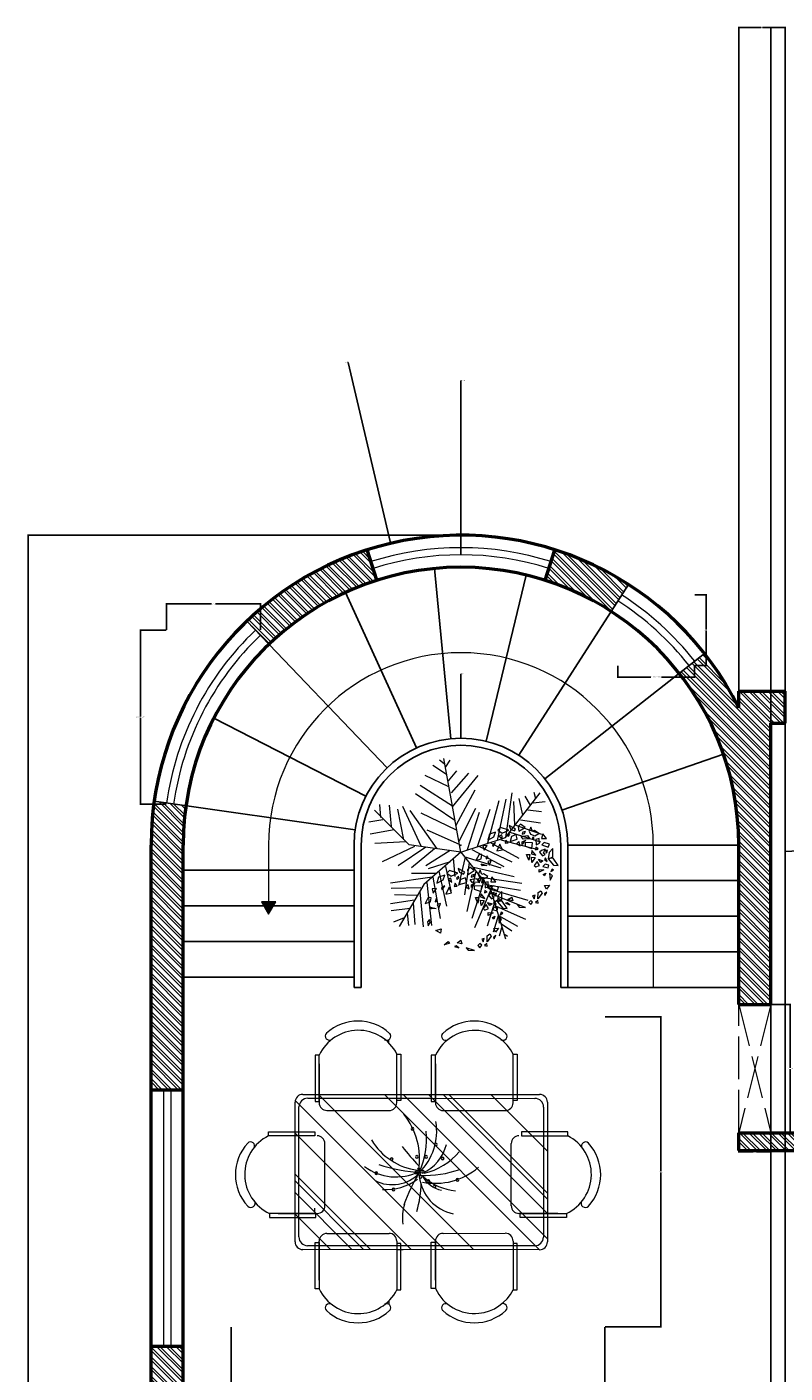
# Model space of a CAD drawing. Units: inches. Extents: x 10696 to 11614, y 5787 to 6498.
# Tile 4 of 9: x 10696 to 10909, y 6120 to 6498. Entities that reach past the tile are written whole.
import ezdxf

# ---------------------------------------------------------------- set-up
doc = ezdxf.new("R2010")
doc.units = ezdxf.units.IN
doc.linetypes.add('ACAD_ISO02W100', pattern=[15, 12, -3])
for name, color, linetype, lineweight in [('A-ANNO-DIMS', 2, 'Continuous', 18), ('A-ANNO-SYMB', 2, 'Continuous', 18), ('A-DOOR', 3, 'Continuous', 25), ('A-FLOR-STRS', 7, 'Continuous', 25), ('A-FURN', 8, 'Continuous', 18), ('A-GLAZ', 4, 'Continuous', 20), ('A-WALL', 7, 'Continuous', 50), ('A-WALL-OVHD', 7, 'ACAD_ISO02W100', 18), ('A-WALL-PATT', 252, 'Continuous', 13), ('L-PLNT', 94, 'Continuous', 13)]:
    doc.layers.add(name, color=color, linetype=linetype, lineweight=lineweight)
doc.styles.get("Standard").update_dxf_attribs({"font": 'arial.ttf'})
doc.dimstyles.get("Standard").update_dxf_attribs({"dimtxt": 0.18, "dimasz": 0.18, "dimexe": 0.18, "dimexo": 0.0625, "dimgap": 0.09, "dimtad": 0, "dimtih": 1, "dimtoh": 1, "dimdec": 4, "dimzin": 0, "dimdsep": 46, "dimtxsty": 'Standard', "dimcen": 0.09, "dimadec": 0, "dimazin": 0, "dimtfac": 1, "dimtdec": 4, "dimtofl": 0, "dimtmove": 0, "dimatfit": 3, "dimfxl": 1, "dimtolj": 1, "dimtzin": 0, "dimarcsym": 0})

# ---------------------------------------------------------------- blocks, each defined once
blk = doc.blocks.new('*U2')
for p, q in [((-8.737, 47.138), (-17.069, 52.711)), ((-10.186, 53.64), (-13.084, 55.962)), ((0, 0), (-10.5, 57)), ((-9.099, 51.782), (-6.563, 55.962)), ((-7.65, 43.423), (-2.578, 49.46)), ((-7.288, 39.707), (-21.778, 46.673)), ((-5.839, 35.992), (4.667, 48.067)), ((-5.114, 27.632), (10.463, 46.673)), ((-3.665, 19.273), (-27.574, 35.527)), ((-5.114, 28.097), (-24.676, 40.636)), ((-2.941, 16.486), (8.652, 37.85)), ((27, 9), (48, 36)), ((27.127, 9.056), (31.112, 35.992)), ((35.096, 32.741), (37.27, 22.524)), ((38.719, 34.134), (41.979, 28.561)), ((44.153, 36.456), (45.239, 32.741)), ((-31.5, 4.5), (-52.5, 25.5)), ((-48.585, 21.131), (-49.309, 29.026)), ((-43.513, 28.561), (-42.427, 15.558)), ((-38.442, 26.239), (-34.819, 7.663)), ((-35.544, 28.097), (-24.314, 3.947)), ((-14.533, 2.09), (-30.834, 25.31)), ((-1.129, 6.734), (9.014, 26.704)), ((10.101, 3.483), (17.708, 26.239)), ((16.259, 5.805), (23.142, 31.348)), ((22.055, 7.198), (27.489, 32.277)), ((31.836, 30.883), (32.561, 16.486)), ((40.53, 25.775), (48.862, 24.846)), ((43.791, 29.954), (51.036, 30.883)), ((-47.498, 19.737), (-55.83, 18.344)), ((-24.314, 23.917), (-2.941, 13.7)), ((3.942, 1.625), (11.187, 24.381)), ((33.285, 16.486), (48.862, 10.913)), ((36.183, 19.737), (48.137, 17.88)), ((-40.615, 13.7), (-55.105, 10.913)), ((-20.691, 13.7), (-1.129, 4.876)), ((0, 0), (27, 9)), ((29.662, 12.307), (48.137, 6.269)), ((-33.37, 6.269), (-52.207, 5.34)), ((-28.299, 3.483), (-47.86, -5.805)), ((-21.416, 3.018), (-38.079, -8.128)), ((0, 0), (-31.5, 4.5)), ((-15.982, 2.09), (-30.11, -9.521)), ((0, 0), (-22.5, -19.5)), ((-6.563, 1.161), (-21.416, -8.128)), ((0, 0), (18, -22.5)), ((6.478, 1.625), (26.04, -8.592)), ((11.187, 3.483), (30.749, -5.805)), ((18.07, 5.805), (35.096, -3.483)), ((24.229, 7.663), (46.688, 1.625)), ((-6.563, -5.805), (-19.967, -9.985)), ((-4.752, -3.483), (-3.665, -14.629)), ((2.493, -3.019), (-1.491, -20.202)), ((1.769, -2.555), (24.229, -9.521)), ((5.029, -6.27), (2.131, -25.775)), ((-17.431, -15.094), (-42.789, -18.809)), ((-15.257, -12.772), (-30.11, -12.772)), ((-17.069, -15.094), (-12.721, -40.172)), ((-13.446, -11.378), (-8.737, -32.741)), ((-9.461, -8.592), (-6.201, -23.453)), ((9.014, -11.378), (3.58, -35.992)), ((7.565, -9.056), (32.198, -14.629)), ((12.274, -15.094), (36.907, -18.809)), ((-24.314, -21.596), (-42.427, -22.06)), ((-22.5, -19.5), (-37.5, -45)), ((-25.038, -23.918), (-22.865, -45.281)), ((-20.691, -18.345), (-17.793, -44.352)), ((14.085, -16.951), (6.478, -40.172)), ((18.07, -22.524), (8.289, -45.745)), ((16.259, -19.738), (36.183, -22.989)), ((18, -22.5), (27, -52.5)), ((18.433, -22.524), (40.53, -29.026)), ((-28.299, -29.026), (-42.789, -31.348)), ((-26.849, -26.24), (-40.253, -25.775)), ((-29.023, -30.884), (-27.936, -43.887)), ((20.244, -30.419), (15.897, -44.816)), ((19.157, -25.311), (38.719, -33.206)), ((-30.834, -34.135), (-42.427, -35.528)), ((-34.457, -39.708), (-40.978, -42.494)), ((-32.646, -36.921), (-31.921, -44.352)), ((22.78, -37.85), (19.519, -48.532)), ((21.331, -32.741), (39.081, -40.636)), ((22.78, -38.314), (34.372, -44.816)), ((24.591, -45.745), (23.142, -50.854)), ((24.591, -43.423), (30.749, -47.603)), ((26.764, -49.925), (28.213, -50.854))]:
    blk.add_line(p, q)
blk = doc.blocks.new('*U3')
for points in [[(-2, 11.66), (-1.6, 10.62), (-0.52, 10.1), (-0.18, 10.62), (-0.79, 10.96)], [(1.24, 12), (0.56, 11.31), (0.76, 10.01), (2.52, 11.05)], [(-5.78, 9.75), (-7.54, 9.23), (-8.01, 7.5), (-6.26, 8.45)], [(-4.43, 11.05), (-5.18, 10.36), (-3.96, 9.49), (-2.07, 10.36)], [(-4.84, 8.63), (-3.83, 7.85), (-4.03, 8.97)], [(-1.94, 9.49), (-2.48, 8.97), (-2.27, 8.54), (-1.8, 9.06)], [(0.02, 9.06), (-1.33, 8.54), (-1.73, 7.16), (0.29, 7.76)], [(1.37, 8.54), (3.13, 8.8), (3.8, 7.85), (1.91, 7.76)], [(2.59, 9.93), (1.84, 9.75), (1.64, 9.23), (2.32, 9.41)], [(4.14, 11.14), (3.6, 10.01), (4, 9.23), (5.22, 8.71), (6.3, 9.41), (5.08, 10.19), (4.61, 10.01)], [(4.61, 8.28), (4.54, 7.76), (4.95, 7.59), (4.95, 8.28)], [(6.43, 7.94), (5.49, 7.68), (5.56, 6.21), (6.5, 6.64)], [(7.45, 9.32), (7.11, 7.94), (8.52, 7.94)], [(-8.14, 6.03), (-9.36, 5.95), (-9.02, 4.73)], [(-5.78, 6.81), (-6.66, 6.21), (-6.52, 5.69)], [(-4.57, 6.38), (-5.45, 4.47), (-3.89, 4.82)], [(-2.88, 7.5), (-3.15, 6.64), (-2.27, 6.72)], [(0.76, 7.16), (0.09, 6.46), (1.1, 5.95)], [(1.71, 6.29), (1.71, 7.07), (2.65, 7.5), (2.11, 6.9)], [(2.52, 6.81), (2.52, 5.86), (4.41, 5.17), (4.61, 6.72)], [(4.41, 4.56), (4.27, 3.7), (5.49, 3.26)], [(5.49, 5.51), (5.42, 4.82), (6.16, 5.08)], [(8.12, 4.99), (7.11, 4.65), (6.5, 4.13), (7.38, 3.09), (8.12, 3.52), (7.65, 3.87)], [(7.85, 6.81), (7.18, 6.21), (9, 5.51), (9.33, 6.38)], [(8.73, 4.73), (8.19, 4.56), (8.39, 3.87), (8.59, 4.04)], [(10.28, 5.17), (9.2, 4.04), (9, 2.31), (10.48, 0.49), (11.76, 0.41), (10.35, 2.48), (9.33, 2.4), (10.28, 2.83)], [(-11.32, 1.79), (-9.83, 2.31), (-9.63, 3.44), (-10.44, 3.52)], [(-8.21, 0.41), (-9.43, 0.32), (-9.83, 0.84)], [(-8.21, 3.09), (-8.48, 2.31), (-7.87, 2.57)], [(-7, 1.79), (-7.94, 1.53), (-7.47, 0.49)], [(3.53, 1.88), (2.86, 3.52), (3.8, 3.52)], [(4.27, 2.74), (5.29, 2.66), (4.41, 1.27)], [(5.83, 1.53), (5.02, 0.41), (5.49, -0.02), (6.5, 0.41)], [(7.51, 1.71), (6.91, 1.27), (6.23, 2.14)], [(8.12, 0.75), (7.51, 0.15), (8.93, -0.28), (9.13, 0.49)], [(8.19, 2.57), (7.92, 2.05), (8.66, 1.53)], [(-10.03, -2.71), (-10.64, -3.31), (-10.44, -4.44), (-9.9, -3.49)], [(7.78, -0.8), (6.43, -1.5), (6.43, -0.72)], [(8.32, -1.75), (7.98, -2.53), (7.58, -2.1)], [(9.33, -1.75), (9.54, -3.74), (10.14, -2.53)], [(10.08, -0.63), (9.74, -1.32), (10.48, -0.89)], [(-8.28, -5.73), (-6.79, -5.3), (-7, -6.51)], [(6.1, -8.94), (6.16, -7.21), (6.91, -6.69), (7.24, -7.38)], [(8.05, -8.07), (8.59, -7.12), (7.92, -7.55)], [(9.33, -5.13), (8.46, -6.25), (7.98, -5.22)], [(-4.84, -8.85), (-4.43, -9.45), (-5.99, -9.8)], [(-2.54, -10.06), (-3.02, -10.23), (-1.8, -10.67)], [(-2.34, -9.2), (-1.26, -8.5), (-0.99, -9.54)], [(0.22, -10.58), (0.83, -11.27), (2.59, -11.36)], [(4.07, -9.45), (3.53, -9.97), (4.07, -10.58), (4.61, -9.89)], [(5.29, -7.98), (4.61, -8.16), (5.02, -8.94)], [(6.03, -9.45), (5.42, -9.97), (6.16, -10.15)]]:
    blk.add_lwpolyline(points, close=True)
blk = doc.blocks.new('A$C6327331B')
for p, q in [((790.8, 678.3), (790.8, 696.4)), ((790.8, 678.3), (790.8, 696.4)), ((1381.3, 692.8), (1381.3, 686.2)), ((1381.3, 692.8), (1381.3, 686.2)), ((410.1, 615.8), (410, 377)), ((410.1, 615.8), (410, 377)), ((431.6, 615.8), (410.1, 615.8)), ((431.6, 615.8), (410.1, 615.8)), ((431.4, 376.9), (431.6, 615.8)), ((431.4, 376.9), (431.6, 615.8)), ((431.5, 571.8), (431.4, 370.8)), ((431.5, 571.8), (431.4, 370.8)), ((831.4, 382.9), (831.6, 621.7)), ((831.4, 382.9), (831.6, 621.7)), ((831.4, 370.6), (831.5, 571.6)), ((831.4, 370.6), (831.5, 571.6)), ((831.6, 621.7), (853, 621.7)), ((831.6, 621.7), (853, 621.7)), ((853, 621.7), (852.9, 382.9)), ((853, 621.7), (852.9, 382.9)), ((1009.3, 615.5), (1009.2, 376.7)), ((1009.3, 615.5), (1009.2, 376.7)), ((1030.7, 615.5), (1009.3, 615.5)), ((1030.7, 615.5), (1009.3, 615.5)), ((1030.6, 376.6), (1030.7, 615.5)), ((1030.6, 376.6), (1030.7, 615.5)), ((1030.7, 571.5), (1030.6, 370.5)), ((1030.7, 571.5), (1030.6, 370.5)), ((1430.6, 382.6), (1430.7, 621.4)), ((1430.6, 382.6), (1430.7, 621.4)), ((1430.6, 370.3), (1430.7, 571.3)), ((1430.6, 370.3), (1430.7, 571.3)), ((1430.7, 621.4), (1452.2, 621.4)), ((1430.7, 621.4), (1452.2, 621.4)), ((1452.2, 621.4), (1452, 382.6)), ((1452.2, 621.4), (1452, 382.6)), ((307.1, -346), (307.5, 374)), ((307.1, -346), (307.5, 374)), ((1075.9, -386.3), (308.5, 383.1)), ((1075.9, -386.3), (308.5, 383.1)), ((327.1, -321), (327.5, 349)), ((347.5, 414), (831.5, 413.8)), ((347.5, 414), (831.5, 413.8)), ((372.5, 394), (831.4, 393.8)), ((372.5, 394), (1009.2, 393.7)), ((410, 377), (431.4, 376.9)), ((410, 377), (431.4, 376.9)), ((1226.3, -386.4), (428, 414)), ((1226.3, -386.4), (428, 414)), ((1567.1, -386.6), (768.8, 413.8)), ((1567.1, -386.6), (768.8, 413.8)), ((852.9, 382.9), (831.4, 382.9)), ((852.9, 382.9), (831.4, 382.9)), ((831.5, 413.8), (1567.5, 413.4)), ((1607.1, -331.3), (864.1, 413.8)), ((1607.1, -331.3), (864.1, 413.8)), ((1607.2, -200.8), (994.4, 413.7)), ((1607.2, -200.8), (994.4, 413.7)), ((1009.2, 413.7), (1567.5, 413.4)), ((1009.2, 393.7), (1542.5, 393.4)), ((1009.2, 376.7), (1030.6, 376.6)), ((1009.2, 376.7), (1030.6, 376.6)), ((1607.2, -125.5), (1069.5, 413.7)), ((1607.2, -125.5), (1069.5, 413.7)), ((1607.2, -95.4), (1099.6, 413.6)), ((1607.2, -95.4), (1099.6, 413.6)), ((1607.3, 120.5), (1315.1, 413.5)), ((1607.3, 120.5), (1315.1, 413.5)), ((1415.7, 413.4), (1415.7, 413.5)), ((1415.7, 413.4), (1415.7, 413.5)), ((1452, 382.6), (1430.6, 382.6)), ((1452, 382.6), (1430.6, 382.6)), ((1587.5, 348.4), (1587.1, -321.6)), ((1607.5, 373.4), (1607.1, -346.6)), ((1607.5, 373.4), (1607.1, -346.6)), ((471.4, 330.8), (791.4, 330.6)), ((471.4, 330.8), (791.4, 330.6)), ((1070.6, 330.5), (1390.6, 330.3)), ((1070.6, 330.5), (1390.6, 330.3)), ((169.9, 221.5), (408.7, 221.6)), ((169.9, 221.5), (408.7, 221.6)), ((169.9, 200.1), (169.9, 221.5)), ((169.9, 200.1), (169.9, 221.5)), ((905.5, -386.3), (307.4, 213.5)), ((905.5, -386.3), (307.4, 213.5)), ((408.7, 221.6), (408.7, 200.2)), ((408.7, 221.6), (408.7, 200.2)), ((1473.3, 221.6), (1473.3, 200.2)), ((1473.3, 221.6), (1473.3, 200.2)), ((1712.1, 221.5), (1473.3, 221.6)), ((1712.1, 221.5), (1473.3, 221.6)), ((1712.1, 200.1), (1712.1, 221.5)), ((1712.1, 200.1), (1712.1, 221.5)), ((408.7, 200.2), (169.9, 200.1)), ((408.7, 200.2), (169.9, 200.1)), ((461.2, -159.8), (461, 160.2)), ((461.2, -159.8), (461, 160.2)), ((1420.8, -159.8), (1420.9, 160.2)), ((1420.8, -159.8), (1420.9, 160.2)), ((1473.3, 200.2), (1712.1, 200.1)), ((1473.3, 200.2), (1712.1, 200.1)), ((695.1, -386.2), (307.3, 2.7)), ((695.1, -386.2), (307.3, 2.7)), ((44.6, -20.2), (44.5, -20.1)), ((44.6, -20.2), (44.5, -20.1)), ((660, -386.1), (307.3, -32.5)), ((660, -386.1), (307.3, -32.5)), ((1837.4, -20.2), (1837.5, -20.1)), ((1837.4, -20.2), (1837.5, -20.1)), ((599.8, -386.1), (307.2, -92.7)), ((599.8, -386.1), (307.2, -92.7)), ((415.1, -199.8), (176.2, -199.9)), ((415.1, -199.8), (176.2, -199.9)), ((176.2, -199.9), (176.2, -221.3)), ((176.2, -199.9), (176.2, -221.3)), ((220.2, -199.9), (421.2, -199.8)), ((220.2, -199.9), (421.2, -199.8)), ((489.6, -386), (307.2, -203.2)), ((489.6, -386), (307.2, -203.2)), ((408.7, -193.6), (408.7, -172.1)), ((408.7, -193.6), (408.7, -172.1)), ((415.1, -221.2), (415.1, -199.8)), ((415.1, -221.2), (415.1, -199.8)), ((1661.8, -199.9), (1460.8, -199.8)), ((1661.8, -199.9), (1460.8, -199.8)), ((1466.9, -221.2), (1466.9, -199.8)), ((1466.9, -221.2), (1466.9, -199.8)), ((1466.9, -199.8), (1705.7, -199.9)), ((1466.9, -199.8), (1705.7, -199.9)), ((1705.7, -199.9), (1705.7, -221.3)), ((1705.7, -199.9), (1705.7, -221.3)), ((176.2, -221.3), (415.1, -221.2)), ((176.2, -221.3), (415.1, -221.2)), ((1705.7, -221.3), (1466.9, -221.2)), ((1705.7, -221.3), (1466.9, -221.2)), ((431.5, -543.7), (431.4, -342.7)), ((431.5, -543.7), (431.4, -342.7)), ((471.4, -302.7), (791.4, -302.5)), ((471.4, -302.7), (791.4, -302.5)), ((831.4, -342.5), (831.5, -543.5)), ((831.4, -342.5), (831.5, -543.5)), ((1030.7, -543.4), (1030.6, -342.4)), ((1030.7, -543.4), (1030.6, -342.4)), ((1070.6, -302.4), (1390.6, -302.2)), ((1070.6, -302.4), (1390.6, -302.2)), ((1430.6, -342.2), (1430.7, -543.2)), ((1430.6, -342.2), (1430.7, -543.2)), ((1567.1, -386.6), (347.1, -386)), ((1567.1, -386.6), (347.1, -386)), ((1542.1, -366.6), (372.1, -366)), ((410.1, -587.7), (410, -348.9)), ((410.1, -587.7), (410, -348.9)), ((410, -348.9), (431.4, -348.9)), ((410, -348.9), (431.4, -348.9)), ((431.4, -348.9), (431.6, -587.7)), ((431.4, -348.9), (431.6, -587.7)), ((831.4, -354.8), (831.6, -593.6)), ((831.4, -354.8), (831.6, -593.6)), ((852.9, -354.8), (831.4, -354.8)), ((852.9, -354.8), (831.4, -354.8)), ((831.5, -385.7), (864.1, -385.7)), ((831.5, -385.7), (864.1, -385.7)), ((853, -593.6), (852.9, -354.8)), ((853, -593.6), (852.9, -354.8)), ((1009.2, -348.6), (1030.6, -348.5)), ((1009.2, -348.6), (1030.6, -348.5)), ((1009.3, -587.4), (1009.2, -348.6)), ((1009.3, -587.4), (1009.2, -348.6)), ((1030.6, -348.5), (1030.7, -587.4)), ((1030.6, -348.5), (1030.7, -587.4)), ((1415.7, -385.3), (1415.7, -385.4)), ((1415.7, -385.3), (1415.7, -385.4)), ((1430.6, -354.5), (1430.7, -593.3)), ((1430.6, -354.5), (1430.7, -593.3)), ((1452, -354.5), (1430.6, -354.5)), ((1452, -354.5), (1430.6, -354.5)), ((1452.2, -593.3), (1452, -354.5)), ((1452.2, -593.3), (1452, -354.5)), ((431.6, -587.7), (410.1, -587.7)), ((431.6, -587.7), (410.1, -587.7)), ((831.6, -593.6), (853, -593.6)), ((831.6, -593.6), (853, -593.6)), ((1030.7, -587.4), (1009.3, -587.4)), ((1030.7, -587.4), (1009.3, -587.4)), ((1430.7, -593.3), (1452.2, -593.3)), ((1430.7, -593.3), (1452.2, -593.3)), ((790.8, -650.2), (790.8, -668.4)), ((790.8, -650.2), (790.8, -668.4)), ((1381.3, -664.7), (1381.3, -658.1)), ((1381.3, -664.7), (1381.3, -658.1))]:
    blk.add_line(p, q)
for centre, radius, start, end in [((631.5, 550.5), 241.3, 47.46915, 132.47205), ((631.5, 550.5), 241.3, 47.46915, 132.47205), ((1230.7, 550.2), 241.3, 47.46915, 132.47205), ((1230.7, 550.2), 241.3, 47.46915, 132.47205), ((633, 521.6), 222.4, 26.76564, 154.93691), ((633, 521.6), 222.4, 26.76564, 154.93691), ((484.3, 714.2), 21.2, 137.64965, 300.34124), ((484.3, 714.2), 21.2, 137.64965, 300.34124), ((779, 714), 21.2, 239.59996, 42.29154), ((779, 714), 21.2, 239.59996, 42.29154), ((1232.2, 521.3), 222.4, 84.42654, 154.93691), ((1232.2, 521.3), 222.4, 84.42654, 154.93691), ((1083.4, 713.9), 21.2, 137.64965, 300.34124), ((1083.4, 713.9), 21.2, 137.64965, 300.34124), ((1232.2, 521.3), 222.4, 26.76564, 84.42654), ((1232.2, 521.3), 222.4, 26.76564, 84.42654), ((1378.1, 713.7), 21.2, 239.59996, 42.29154), ((1378.1, 713.7), 21.2, 239.59996, 42.29154), ((347.5, 374), 40, 89.9706, 179.9706), ((347.5, 374), 40, 89.9706, 179.9706), ((372.5, 349), 45, 89.9706, 179.9706), ((471.4, 370.8), 40, 179.9706, 269.9706), ((471.4, 370.8), 40, 179.9706, 269.9706), ((791.4, 370.6), 40, 269.9706, 359.9706), ((791.4, 370.6), 40, 269.9706, 359.9706), ((1070.6, 370.5), 40, 179.9706, 269.9706), ((1070.6, 370.5), 40, 179.9706, 269.9706), ((1390.6, 370.3), 40, 269.9706, 359.9706), ((1390.6, 370.3), 40, 269.9706, 359.9706), ((1542.5, 348.4), 45, 359.9706, 89.9706), ((1567.5, 373.4), 40, 359.9706, 89.9706), ((1567.5, 373.4), 40, 359.9706, 89.9706), ((574.1, 79.9), 374.6, 351.24958, 38.23328), ((912.6, 235.7), 6.91, 0, 180), ((912.6, 235.7), 6.91, 180, 0), ((737.8, 225), 299.2, 314.48606, 9.37622), ((586.4, 182.9), 398.1, 335.08876, 5.96372), ((241.3, 0.1), 241.3, 137.52795, 222.53085), ((270.2, 1.6), 222.4, 116.82445, 244.99571), ((270.2, 1.6), 222.4, 116.82445, 244.99571), ((77.6, 147.4), 21.2, 329.65876, 132.35035), ((77.6, 147.4), 21.2, 329.65876, 132.35035), ((421, 160.2), 40, 0.0294, 90.0294), ((421, 160.2), 40, 0.0294, 90.0294), ((983.2, 350.8), 331, 211.31505, 262.13779), ((2460.3, 1443.6), 2062.1, 219.04877, 222.6799), ((873.8, 207.8), 219.3, 294.09558, 346.29534), ((1033, 155.9), 6.91, 0, 180), ((1033, 155.9), 6.91, 180, 0), ((1460.9, 160.2), 40, 89.9706, 179.9706), ((1460.9, 160.2), 40, 89.9706, 179.9706), ((1611.7, 1.6), 222.4, 295.00429, 63.17555), ((1611.7, 1.6), 222.4, 295.00429, 63.17555), ((1804.4, 147.4), 21.2, 47.64965, 210.34124), ((1804.4, 147.4), 21.2, 47.64965, 210.34124), ((1640.7, 0.1), 241.3, 317.46915, 42.47205), ((1640.7, 0.1), 241.3, 317.46915, 42.47205), ((805, 79.9), 6.91, 0, 180), ((805, 79.9), 6.91, 180, 0), ((934.8, 91.3), 6.91, 0, 180), ((934.8, 91.3), 6.91, 180, 0), ((897.1, 334.6), 335.6, 283.04524, 319.77663), ((982.3, 91.3), 6.91, 0, 180), ((982.3, 91.3), 6.91, 180, 0), ((1067.8, 83.7), 6.91, 0, 180), ((1067.8, 83.7), 6.91, 180, 0), ((826.9, 258.5), 270.1, 233.32313, 295.76326), ((725.8, 7.7), 6.91, 0, 180), ((725.8, 7.7), 6.91, 180, 0), ((807.8, 143), 194.5, 242.99086, 315.91017), ((985.1, 750.7), 739.8, 250.5249, 267.82437), ((1747.6, -469.5), 933.6, 148.98728, 160.36101), ((931.7, 11.5), 6.91, 0, 180), ((931.7, 11.5), 6.91, 180, 0), ((944.3, 26.7), 6.91, 0, 180), ((944.3, 26.7), 6.91, 180, 0), ((947.5, 3.9), 6.91, 0, 180), ((947.5, 3.9), 6.91, 180, 0), ((970.7, 574.8), 578.8, 268.32856, 288.729), ((966.5, 15.3), 6.91, 0, 180), ((966.5, 15.3), 6.91, 180, 0), ((1030.3, 292.7), 337.4, 258.55155, 310.98153), ((776.7, 191.6), 268.2, 265.87406, 306.95584), ((814.5, -75.9), 6.91, 0, 180), ((392.7, -33), 564.4, 343.85612, 359.11051), ((953.8, -11.3), 6.91, 0, 180), ((953.8, -11.3), 6.91, 180, 0), ((1167.7, 15.7), 221.9, 186.99045, 258.02836), ((1090.6, 62.7), 145.4, 208.89012, 258.45792), ((1166.2, 212.9), 298.2, 228.7581, 263.8624), ((995, -34.1), 6.91, 0, 180), ((995, -34.1), 6.91, 180, 0), ((1026.7, -60.7), 6.91, 0, 180), ((1026.7, -60.7), 6.91, 180, 0), ((1143.8, -26.5), 6.91, 0, 180), ((1143.8, -26.5), 6.91, 180, 0), ((79, -146.7), 22.5, 226.37763, 29.88821), ((79, -146.7), 22.5, 226.37763, 29.88821), ((814.5, -75.9), 6.91, 180, 0), ((1803, -146.7), 22.5, 150.11179, 313.62237), ((1803, -146.7), 22.5, 150.11179, 313.62237), ((421.2, -159.8), 40, 270.0294, 0.0294), ((421.2, -159.8), 40, 270.0294, 0.0294), ((1112.9, -226), 252.6, 162.94564, 186.48138), ((1460.8, -159.8), 40, 179.9706, 269.9706), ((1460.8, -159.8), 40, 179.9706, 269.9706), ((347.1, -346), 40, 179.9706, 269.9706), ((347.1, -346), 40, 179.9706, 269.9706), ((372.1, -321), 45, 179.9706, 269.9706), ((471.4, -342.7), 40, 90.0294, 180.0294), ((471.4, -342.7), 40, 90.0294, 180.0294), ((791.4, -342.5), 40, 0.0294, 90.0294), ((791.4, -342.5), 40, 0.0294, 90.0294), ((1070.6, -342.4), 40, 90.0294, 180.0294), ((1070.6, -342.4), 40, 90.0294, 180.0294), ((1390.6, -342.2), 40, 0.0294, 90.0294), ((1390.6, -342.2), 40, 0.0294, 90.0294), ((1542.1, -321.6), 45, 269.9706, 359.9706), ((1567.1, -346.6), 40, 269.9706, 359.9706), ((1567.1, -346.6), 40, 269.9706, 359.9706), ((633, -493.5), 222.4, 205.06309, 333.23436), ((633, -493.5), 222.4, 205.06309, 333.23436), ((1232.2, -493.2), 222.4, 205.06309, 275.57346), ((1232.2, -493.2), 222.4, 205.06309, 275.57346), ((1232.2, -493.2), 222.4, 275.57346, 333.23436), ((1232.2, -493.2), 222.4, 275.57346, 333.23436), ((484.3, -686.1), 21.2, 59.65876, 222.35035), ((484.3, -686.1), 21.2, 59.65876, 222.35035), ((779, -686), 21.2, 317.70846, 120.40004), ((779, -686), 21.2, 317.70846, 120.40004), ((1083.4, -685.8), 21.2, 59.65876, 222.35035), ((1083.4, -685.8), 21.2, 59.65876, 222.35035), ((1378.1, -685.6), 21.2, 317.70846, 120.40004), ((1378.1, -685.6), 21.2, 317.70846, 120.40004), ((631.5, -522.4), 241.3, 227.52795, 312.53085), ((631.5, -522.4), 241.3, 227.52795, 312.53085), ((1230.7, -522.1), 241.3, 227.52795, 312.53085), ((1230.7, -522.1), 241.3, 227.52795, 312.53085)]:
    blk.add_arc(centre, radius, start, end)
at = {"width": 0.8, "flags": 9}
for tag in ['XSIZE', 'YSIZE']:
    blk.add_attdef(tag, (945.2, 11.4), '', height=0.23, rotation=180, dxfattribs=at)
blk = doc.blocks.new('DOOR-SINGLE-36-KITCHEN')
blk.add_line((0, 36), (0, 0))
blk.add_arc((0, 36), 36, 270, 0)
blk = doc.blocks.new('WIN-GLAZ-72')
for p, q in [((0, 72), (0, 0)), ((2, 72), (2, 0))]:
    blk.add_line(p, q)
blk = doc.blocks.new('WIN-ARC-CROWN')
for radius in [83.5, 81.5]:
    blk.add_arc((25.29, -77.67), radius, 72.3705, 107.6295)
blk = doc.blocks.new('WIN-ARC-WEST')
for radius in [83.5, 81.5]:
    blk.add_arc((82.66, -11.5), radius, 133.6902, 171.8873)
blk = doc.blocks.new('WIN-ARC-EAST')
for radius in [83.5, 81.5]:
    blk.add_arc((-44.03, -50.4), radius, 38.1972, 57.2958)
blk = doc.blocks.new('OPENING-OVHD-36X9')
for p, q in [((0, 0), (0, 36)), ((9, 36), (0, 0)), ((0, 36), (9, 0)), ((9, 0), (9, 36))]:
    blk.add_line(p, q)
blk = doc.blocks.new('STAIR-HANDRAIL-RETURN')
for p, q in [((0, 0), (0, 40)), ((60, 0), (60, 40)), ((2, 0), (0, 0)), ((58, 0), (60, 0))]:
    blk.add_line(p, q)
blk.add_lwpolyline([(2, 0), (2, 40, -1), (58, 40), (58, 0)], format="xyb")
blk.add_arc((30, 40), 30, 0, 180)
blk = doc.blocks.new('*D36')
at = {"layer": 'A-ANNO-DIMS', "color": 0, "lineweight": -2, "transparency": 16777216}
for p, q in [((10753.44, 6132.46), (10753.44, 6116.62)), ((10858.3, 6132.46), (10858.3, 6116.62)), ((10753.62, 6116.8), (10804.52, 6116.8)), ((10858.12, 6116.8), (10807.22, 6116.8))]:
    blk.add_line(p, q, dxfattribs=at)
at = {"layer": 'A-ANNO-DIMS', "color": 0, "transparency": 16777216}
for points in [[(10753.62, 6116.83), (10753.62, 6116.77), (10753.44, 6116.8)], [(10858.12, 6116.83), (10858.12, 6116.77), (10858.3, 6116.8)]]:
    blk.add_solid(points, dxfattribs=at)
at = {"layer": 'Defpoints', "color": 0, "transparency": 16777216}
for p in [(10753.44, 6132.52), (10858.3, 6132.52), (10858.3, 6116.8)]:
    blk.add_point(p, dxfattribs=at)
at = {"layer": 'A-ANNO-DIMS', "color": 0, "transparency": 16777216, "insert": (10805.87, 6116.8), "char_height": 0.18, "attachment_point": 5}
blk.add_mtext('\\A1;DINING SET 105 TYP.', dxfattribs=at)
blk = doc.blocks.new('*D37')
at = {"layer": 'A-ANNO-DIMS', "color": 0, "lineweight": -2, "transparency": 16777216}
for p, q in [((10858.36, 6219.59), (10874.21, 6219.59)), ((10874.03, 6219.41), (10874.03, 6176.24)), ((10874.03, 6132.7), (10874.03, 6175.88)), ((10858.36, 6132.52), (10874.21, 6132.52))]:
    blk.add_line(p, q, dxfattribs=at)
at = {"layer": 'A-ANNO-DIMS', "color": 0, "transparency": 16777216}
for points in [[(10874, 6219.41), (10874.06, 6219.41), (10874.03, 6219.59)], [(10874, 6132.7), (10874.06, 6132.7), (10874.03, 6132.52)]]:
    blk.add_solid(points, dxfattribs=at)
at = {"layer": 'Defpoints', "color": 0, "transparency": 16777216}
for p in [(10858.3, 6219.59), (10874.03, 6219.59), (10858.3, 6132.52)]:
    blk.add_point(p, dxfattribs=at)
at = {"layer": 'A-ANNO-DIMS', "color": 0, "transparency": 16777216, "insert": (10874.03, 6176.06), "char_height": 0.18, "attachment_point": 5}
blk.add_mtext('\\A1;87 TYP.', dxfattribs=at)
blk = doc.blocks.new('*D54')
at = {"layer": 'A-ANNO-DIMS', "color": 0, "lineweight": -2, "transparency": 16777216}
for p, q in [((10735.19, 6328.25), (10727.74, 6328.25)), ((10727.92, 6328.07), (10727.92, 6303.99)), ((10727.92, 6279.55), (10727.92, 6303.62)), ((10735.19, 6279.37), (10727.74, 6279.37))]:
    blk.add_line(p, q, dxfattribs=at)
at = {"layer": 'A-ANNO-DIMS', "color": 0, "transparency": 16777216}
for points in [[(10727.89, 6328.07), (10727.95, 6328.07), (10727.92, 6328.25)], [(10727.89, 6279.55), (10727.95, 6279.55), (10727.92, 6279.37)]]:
    blk.add_solid(points, dxfattribs=at)
at = {"layer": 'Defpoints', "color": 0, "transparency": 16777216}
for p in [(10727.92, 6328.25), (10735.25, 6328.25), (10735.25, 6279.37)]:
    blk.add_point(p, dxfattribs=at)
at = {"layer": 'A-ANNO-DIMS', "color": 0, "transparency": 16777216, "insert": (10727.92, 6303.81), "char_height": 0.18, "attachment_point": 5}
blk.add_mtext('\\A1;CURVED LIGHT 49 TYP.', dxfattribs=at)
blk = doc.blocks.new('*D55')
at = {"layer": 'A-ANNO-DIMS', "color": 0, "lineweight": -2, "transparency": 16777216}
for p, q in [((10735.25, 6328.31), (10735.25, 6335.76)), ((10735.43, 6335.58), (10747.9, 6335.58)), ((10761.44, 6335.58), (10748.96, 6335.58)), ((10761.62, 6328.31), (10761.62, 6335.76))]:
    blk.add_line(p, q, dxfattribs=at)
at = {"layer": 'A-ANNO-DIMS', "color": 0, "transparency": 16777216}
for points in [[(10735.43, 6335.61), (10735.43, 6335.55), (10735.25, 6335.58)], [(10761.44, 6335.61), (10761.44, 6335.55), (10761.62, 6335.58)]]:
    blk.add_solid(points, dxfattribs=at)
at = {"layer": 'Defpoints', "color": 0, "transparency": 16777216}
for p in [(10761.62, 6335.58), (10735.25, 6328.25), (10761.62, 6328.25)]:
    blk.add_point(p, dxfattribs=at)
at = {"layer": 'A-ANNO-DIMS', "color": 0, "transparency": 16777216, "insert": (10748.43, 6335.58), "char_height": 0.18, "attachment_point": 5}
blk.add_mtext('\\A1;26 TYP.', dxfattribs=at)
blk = doc.blocks.new('*D56')
at = {"layer": 'A-ANNO-DIMS', "color": 0, "lineweight": -2, "transparency": 16777216}
for p, q in [((10861.95, 6318.2), (10861.95, 6314.85)), ((10883.53, 6318.2), (10883.53, 6314.85)), ((10862.13, 6315.03), (10871.24, 6315.03)), ((10883.35, 6315.03), (10874.24, 6315.03))]:
    blk.add_line(p, q, dxfattribs=at)
at = {"layer": 'A-ANNO-DIMS', "color": 0, "transparency": 16777216}
for points in [[(10862.13, 6315.06), (10862.13, 6315), (10861.95, 6315.03)], [(10883.35, 6315.06), (10883.35, 6315), (10883.53, 6315.03)]]:
    blk.add_solid(points, dxfattribs=at)
at = {"layer": 'Defpoints', "color": 0, "transparency": 16777216}
for p in [(10861.95, 6318.27), (10883.53, 6318.27), (10883.53, 6315.03)]:
    blk.add_point(p, dxfattribs=at)
at = {"layer": 'A-ANNO-DIMS', "color": 0, "transparency": 16777216, "insert": (10872.74, 6315.03), "char_height": 0.18, "attachment_point": 5}
blk.add_mtext('\\A1;CURVED LIGHT 22 TYP.', dxfattribs=at)
blk = doc.blocks.new('*D57')
at = {"layer": 'A-ANNO-DIMS', "color": 0, "lineweight": -2, "transparency": 16777216}
for p, q in [((10883.6, 6338.13), (10886.95, 6338.13)), ((10886.77, 6337.95), (10886.77, 6328.38)), ((10886.77, 6318.45), (10886.77, 6328.02)), ((10883.6, 6318.27), (10886.95, 6318.27))]:
    blk.add_line(p, q, dxfattribs=at)
at = {"layer": 'A-ANNO-DIMS', "color": 0, "transparency": 16777216}
for points in [[(10886.74, 6337.95), (10886.8, 6337.95), (10886.77, 6338.13)], [(10886.74, 6318.45), (10886.8, 6318.45), (10886.77, 6318.27)]]:
    blk.add_solid(points, dxfattribs=at)
at = {"layer": 'Defpoints', "color": 0, "transparency": 16777216}
for p in [(10883.53, 6338.13), (10886.77, 6338.13), (10883.53, 6318.27)]:
    blk.add_point(p, dxfattribs=at)
at = {"layer": 'A-ANNO-DIMS', "color": 0, "transparency": 16777216, "insert": (10886.77, 6328.2), "char_height": 0.18, "attachment_point": 5}
blk.add_mtext('\\A1;20 TYP.', dxfattribs=at)
blk = doc.blocks.new('*D64')
at = {"layer": 'A-ANNO-DIMS', "color": 0, "lineweight": -2, "transparency": 16777216}
for p, q in [((10904.98, 6223.07), (10910.49, 6223.07)), ((10910.31, 6222.89), (10910.31, 6205.25)), ((10910.31, 6187.25), (10910.31, 6204.89)), ((10904.98, 6187.07), (10910.49, 6187.07))]:
    blk.add_line(p, q, dxfattribs=at)
at = {"layer": 'A-ANNO-DIMS', "color": 0, "transparency": 16777216}
for points in [[(10910.28, 6222.89), (10910.34, 6222.89), (10910.31, 6223.07)], [(10910.28, 6187.25), (10910.34, 6187.25), (10910.31, 6187.07)]]:
    blk.add_solid(points, dxfattribs=at)
at = {"layer": 'Defpoints', "color": 0, "transparency": 16777216}
for p in [(10904.91, 6223.07), (10910.31, 6223.07), (10904.91, 6187.07)]:
    blk.add_point(p, dxfattribs=at)
at = {"layer": 'A-ANNO-DIMS', "color": 0, "transparency": 16777216, "insert": (10910.31, 6205.07), "char_height": 0.18, "attachment_point": 5}
blk.add_mtext('\\A1;OPENING 36 TYP.', dxfattribs=at)
blk = doc.blocks.new('*D65')
at = {"layer": 'A-ANNO-DIMS', "color": 0, "lineweight": -2, "transparency": 16777216}
for p, q in [((10895.91, 6187.01), (10895.91, 6181.49)), ((10904.91, 6187.01), (10904.91, 6181.49)), ((10896.09, 6181.67), (10899.95, 6181.67)), ((10904.73, 6181.67), (10900.87, 6181.67))]:
    blk.add_line(p, q, dxfattribs=at)
at = {"layer": 'A-ANNO-DIMS', "color": 0, "transparency": 16777216}
for points in [[(10896.09, 6181.7), (10896.09, 6181.64), (10895.91, 6181.67)], [(10904.73, 6181.7), (10904.73, 6181.64), (10904.91, 6181.67)]]:
    blk.add_solid(points, dxfattribs=at)
at = {"layer": 'Defpoints', "color": 0, "transparency": 16777216}
for p in [(10895.91, 6187.07), (10904.91, 6187.07), (10904.91, 6181.67)]:
    blk.add_point(p, dxfattribs=at)
at = {"layer": 'A-ANNO-DIMS', "color": 0, "transparency": 16777216, "insert": (10900.41, 6181.67), "char_height": 0.18, "attachment_point": 5}
blk.add_mtext('\\A1;9 TYP.', dxfattribs=at)
blk = doc.blocks.new('*D71')
at = {"layer": 'A-ANNO-DIMS', "color": 0, "lineweight": -2, "transparency": 16777216}
for p, q in [((10816.99, 6354.91), (10696.18, 6354.91)), ((10696.36, 6354.73), (10696.36, 6106.17)), ((10696.36, 5857.25), (10696.36, 6105.81)), ((10730.85, 5857.07), (10696.18, 5857.07))]:
    blk.add_line(p, q, dxfattribs=at)
at = {"layer": 'A-ANNO-DIMS', "color": 0, "transparency": 16777216}
for points in [[(10696.33, 6354.73), (10696.39, 6354.73), (10696.36, 6354.91)], [(10696.33, 5857.25), (10696.39, 5857.25), (10696.36, 5857.07)]]:
    blk.add_solid(points, dxfattribs=at)
at = {"layer": 'Defpoints', "color": 0, "transparency": 16777216}
for p in [(10696.36, 6354.91), (10817.05, 6354.91), (10730.91, 5857.07)]:
    blk.add_point(p, dxfattribs=at)
at = {"layer": 'A-ANNO-DIMS', "color": 0, "transparency": 16777216, "insert": (10696.36, 6105.99), "char_height": 0.18, "attachment_point": 5}
blk.add_mtext('\\A1;497.8', dxfattribs=at)
blk = doc.blocks.new('*D97')
at = {"layer": 'A-ANNO-DIMS', "color": 0, "lineweight": -2, "transparency": 16777216}
for p, q in [((10895.91, 6311.13), (10895.91, 6497.62)), ((10896.09, 6497.44), (10902.2, 6497.44)), ((10908.73, 6497.44), (10902.62, 6497.44)), ((10908.91, 6311.13), (10908.91, 6497.62))]:
    blk.add_line(p, q, dxfattribs=at)
at = {"layer": 'A-ANNO-DIMS', "color": 0, "transparency": 16777216}
for points in [[(10896.09, 6497.47), (10896.09, 6497.41), (10895.91, 6497.44)], [(10908.73, 6497.47), (10908.73, 6497.41), (10908.91, 6497.44)]]:
    blk.add_solid(points, dxfattribs=at)
at = {"layer": 'Defpoints', "color": 0, "transparency": 16777216}
for p in [(10908.91, 6497.44), (10895.91, 6311.07), (10908.91, 6311.07)]:
    blk.add_point(p, dxfattribs=at)
at = {"layer": 'A-ANNO-DIMS', "color": 0, "transparency": 16777216, "insert": (10902.41, 6497.44), "char_height": 0.18, "attachment_point": 5}
blk.add_mtext('\\A1;13', dxfattribs=at)
blk = doc.blocks.new('*D100')
at = {"layer": 'A-ANNO-DIMS', "color": 0, "lineweight": -2, "transparency": 16777216}
for p, q in [((10904.91, 6078.13), (10904.91, 6497.62)), ((10905.09, 6497.44), (10906.76, 6497.44)), ((10908.73, 6497.44), (10907.07, 6497.44)), ((10908.91, 6078.13), (10908.91, 6497.62))]:
    blk.add_line(p, q, dxfattribs=at)
at = {"layer": 'A-ANNO-DIMS', "color": 0, "transparency": 16777216}
for points in [[(10905.09, 6497.47), (10905.09, 6497.41), (10904.91, 6497.44)], [(10908.73, 6497.47), (10908.73, 6497.41), (10908.91, 6497.44)]]:
    blk.add_solid(points, dxfattribs=at)
at = {"layer": 'Defpoints', "color": 0, "transparency": 16777216}
for p in [(10908.91, 6497.44), (10904.91, 6078.07), (10908.91, 6078.07)]:
    blk.add_point(p, dxfattribs=at)
at = {"layer": 'A-ANNO-DIMS', "color": 0, "transparency": 16777216, "insert": (10906.91, 6497.44), "char_height": 0.18, "attachment_point": 5}
blk.add_mtext('\\A1;4', dxfattribs=at)
blk = doc.blocks.new('*D101')
at = {"layer": 'A-ANNO-DIMS', "color": 0, "lineweight": -2, "transparency": 16777216}
for p, q in [((10786.08, 6403.42), (10786.26, 6403.42)), ((10786.26, 6403.42), (10798.09, 6352.76)), ((10817.82, 6267.87), (10818, 6267.87)), ((10817.91, 6267.78), (10817.91, 6267.96))]:
    blk.add_line(p, q, dxfattribs=at)
at = {"layer": 'A-ANNO-DIMS', "color": 0, "transparency": 16777216}
blk.add_solid([(10798.12, 6352.77), (10798.06, 6352.76), (10798.13, 6352.59)], dxfattribs=at)
at = {"layer": 'Defpoints', "color": 0, "transparency": 16777216}
for p in [(10798.13, 6352.59), (10817.91, 6267.87)]:
    blk.add_point(p, dxfattribs=at)
at = {"layer": 'A-ANNO-DIMS', "color": 0, "transparency": 16777216, "insert": (10785.77, 6403.42), "char_height": 0.18, "attachment_point": 5}
blk.add_mtext('\\A1;R87', dxfattribs=at)
blk = doc.blocks.new('*D104')
at = {"layer": 'A-ANNO-DIMS', "color": 0, "lineweight": -2, "transparency": 16777216}
for p, q in [((10818.09, 6315.87), (10817.91, 6315.87)), ((10817.91, 6315.87), (10817.91, 6298.05)), ((10817.82, 6267.87), (10818, 6267.87)), ((10817.91, 6267.78), (10817.91, 6267.96))]:
    blk.add_line(p, q, dxfattribs=at)
at = {"layer": 'A-ANNO-DIMS', "color": 0, "transparency": 16777216}
blk.add_solid([(10817.88, 6298.05), (10817.94, 6298.05), (10817.91, 6297.87)], dxfattribs=at)
at = {"layer": 'Defpoints', "color": 0, "transparency": 16777216}
for p in [(10817.91, 6297.87), (10817.91, 6267.87)]:
    blk.add_point(p, dxfattribs=at)
at = {"layer": 'A-ANNO-DIMS', "color": 0, "transparency": 16777216, "insert": (10818.4, 6315.87), "char_height": 0.18, "attachment_point": 5}
blk.add_mtext('\\A1;R30', dxfattribs=at)
blk = doc.blocks.new('*D106')
at = {"layer": 'A-ANNO-DIMS', "color": 0, "lineweight": -2, "transparency": 16777216}
for p, q in [((10818.09, 6398.27), (10817.91, 6398.27)), ((10817.91, 6398.27), (10817.91, 6349.55)), ((10817.82, 6267.87), (10818, 6267.87)), ((10817.91, 6267.78), (10817.91, 6267.96))]:
    blk.add_line(p, q, dxfattribs=at)
at = {"layer": 'A-ANNO-DIMS', "color": 0, "transparency": 16777216}
blk.add_solid([(10817.88, 6349.55), (10817.94, 6349.55), (10817.91, 6349.37)], dxfattribs=at)
at = {"layer": 'Defpoints', "color": 0, "transparency": 16777216}
for p in [(10817.91, 6349.37), (10817.91, 6267.87)]:
    blk.add_point(p, dxfattribs=at)
at = {"layer": 'A-ANNO-DIMS', "color": 0, "transparency": 16777216, "insert": (10818.7, 6398.27), "char_height": 0.18, "attachment_point": 5}
blk.add_mtext('\\A1;3X R81.5', dxfattribs=at)

msp = doc.modelspace()

# ---------------------------------------------------------------- hatches: boundary and pattern name
at = {"layer": 'A-ANNO-SYMB'}
h = msp.add_hatch(color=256, dxfattribs=at)
h.dxf.hatch_style = 1
h.paths.add_polyline_path([(10765.904, 6251.921), (10761.922, 6251.921), (10763.913, 6248.473)])
at = {"layer": 'A-WALL-PATT'}
h = msp.add_hatch(dxfattribs=at)
h.set_pattern_fill('ANSI32', color=256, scale=0.2, angle=90)
h.paths.add_polyline_path([(10767.913, 5961.07), (10739.913, 5961.07), (10739.913, 6001.333), (10730.913, 6001.333), (10730.913, 5887.07), (10739.913, 5887.07), (10739.913, 5952.07), (10767.913, 5952.07)])
h.paths.add_polyline_path([(10739.913, 6127.055), (10730.913, 6127.055), (10730.913, 6073.333), (10739.913, 6073.333)])
h.paths.add_polyline_path([(10739.913, 6267.869, -0.035413), (10740.694, 6278.876), (10731.784, 6280.146, 0.035413), (10730.913, 6267.869), (10730.913, 6199.055), (10739.913, 6199.055)])
h.paths.add_polyline_path([(10794.29, 6342.205), (10791.564, 6350.783, 0.1142038), (10757.817, 6330.777), (10764.034, 6324.269, -0.1142038)])
h.paths.add_polyline_path([(10844.262, 6350.783), (10841.536, 6342.205, -0.065871), (10860.057, 6333.503), (10864.919, 6341.077, 0.065871)])
h.paths.add_polyline_path([(10908.913, 6311.07), (10895.913, 6311.07), (10895.913, 6306.404, 0.0519949), (10886.285, 6321.667), (10879.212, 6316.101, -0.1682272), (10895.913, 6267.869), (10895.913, 6223.07), (10904.913, 6223.07), (10904.913, 6302.07), (10908.913, 6302.07)])
h.paths.add_polyline_path([(11057.913, 6311.07), (10944.913, 6311.07), (10944.913, 6302.07), (11048.913, 6302.07), (11048.913, 6273.514), (11057.913, 6273.514)])
h.paths.add_polyline_path([(11057.913, 6225.514), (11048.913, 6225.514), (11048.913, 6187.07), (10988.913, 6187.07), (10988.913, 6182.07), (11048.913, 6182.07), (11048.913, 6164.07), (11057.913, 6164.07)])
h.paths.add_polyline_path([(10952.913, 6187.07), (10895.913, 6187.07), (10895.913, 6182.07), (10948.913, 6182.07), (10948.913, 6113.07), (10952.913, 6113.07), (10952.913, 6117.07), (11048.913, 6117.07), (11048.913, 6099.07), (11057.913, 6099.07), (11057.913, 6140.07), (11048.913, 6140.07), (11048.913, 6122.07), (10952.913, 6122.07)])
h.paths.add_polyline_path([(11057.913, 6075.07), (11048.913, 6075.07), (11048.913, 6057.07), (10952.913, 6057.07), (10952.913, 6083.07), (10944.913, 6083.07), (10944.913, 6078.07), (10948.913, 6078.07), (10948.913, 6052.07), (11048.913, 6052.07), (11048.913, 6028.07), (11057.913, 6028.07)])
h.paths.add_polyline_path([(11057.913, 5992.07), (11048.913, 5992.07), (11048.913, 5896.07), (11000.913, 5896.07), (11000.913, 5887.07), (11057.913, 5887.07)])
h.paths.add_polyline_path([(10952.913, 5896.07), (10904.913, 5896.07), (10904.913, 6078.07), (10908.913, 6078.07), (10908.913, 6083.07), (10899.913, 6083.07), (10899.913, 5961.07), (10891.913, 5961.07), (10891.913, 5952.07), (10895.913, 5952.07), (10895.913, 5887.07), (10952.913, 5887.07)])
h.paths.add_polyline_path([(10843.913, 5961.07), (10815.913, 5961.07), (10815.913, 5952.07), (10843.913, 5952.07)])

# ---------------------------------------------------------------- linework, layer by layer
at = {"layer": 'A-ANNO-SYMB'}
for p, q in [((10763.913, 6267.869), (10763.913, 6267.869)), ((10763.913, 6267.869), (10763.913, 6251.921)), ((10871.913, 6267.869), (10871.913, 6227.869))]:
    msp.add_line(p, q, dxfattribs=at)
msp.add_lwpolyline([(10763.913, 6248.473), (10765.904, 6251.921), (10761.922, 6251.921)], close=True, dxfattribs=at)
msp.add_arc((10817.913, 6267.869), 54, 0, 180, dxfattribs=at)
at = {"layer": 'A-FLOR-STRS'}
for p, q in [((10815.041, 6297.731), (10810.447, 6345.51)), ((10824.97, 6297.027), (10836.261, 6343.68)), ((10834.122, 6293.113), (10864.919, 6341.077)), ((10805.429, 6295.147), (10785.453, 6338.794)), ((10797.19, 6289.561), (10757.817, 6330.777)), ((10841.49, 6286.42), (10886.285, 6321.667)), ((10791.233, 6281.587), (10748.545, 6303.536)), ((10846.262, 6277.684), (10891.62, 6293.39)), ((10788.213, 6272.102), (10731.784, 6280.146)), ((10847.913, 6267.869), (10895.913, 6267.869)), ((10787.913, 6260.772), (10739.913, 6260.772)), ((10847.913, 6257.869), (10895.913, 6257.869)), ((10762.586, 6250.772), (10739.913, 6250.772)), ((10787.913, 6250.772), (10765.24, 6250.772)), ((10847.913, 6247.869), (10895.913, 6247.869)), ((10787.913, 6240.772), (10739.913, 6240.772)), ((10847.913, 6237.869), (10895.913, 6237.869)), ((10787.913, 6230.772), (10739.913, 6230.772)), ((10847.913, 6227.869), (10895.913, 6227.869))]:
    msp.add_line(p, q, dxfattribs=at)
at = {"layer": 'A-WALL'}
for p, q in [((10794.29, 6342.205), (10791.564, 6350.783)), ((10841.536, 6342.205), (10844.262, 6350.783)), ((10895.913, 6311.07), (10908.913, 6311.07)), ((10895.913, 6306.404), (10895.913, 6311.07)), ((10908.913, 6302.07), (10908.913, 6311.07)), ((10904.913, 6302.07), (10908.913, 6302.07)), ((10904.913, 6223.07), (10904.913, 6302.07)), ((10730.913, 5857.07), (10730.913, 6267.869)), ((10739.913, 5961.07), (10739.913, 6267.869)), ((10895.913, 6223.07), (10895.913, 6267.869)), ((10895.913, 6223.07), (10904.913, 6223.07)), ((10739.913, 6199.055), (10730.913, 6199.055)), ((10895.913, 6187.07), (10952.913, 6187.07)), ((10895.913, 6182.07), (10895.913, 6187.07)), ((10895.913, 6182.07), (10948.913, 6182.07)), ((10739.913, 6127.055), (10730.913, 6127.055))]:
    msp.add_line(p, q, dxfattribs=at)
for radius, start in [(87, 26.29156), (78, 0)]:
    msp.add_arc((10817.913, 6267.869), radius, start, 180, dxfattribs=at)

# ---------------------------------------------------------------- block references
at = {"layer": 'A-DOOR'}
msp.add_blockref('DOOR-SINGLE-36-KITCHEN', (10908.913, 6266.07), dxfattribs=at)
at = {"layer": 'A-FLOR-STRS'}
msp.add_blockref('STAIR-HANDRAIL-RETURN', (10787.913, 6227.869), dxfattribs=at)
at = {"layer": 'A-FURN', "xscale": 0.0544898626987332, "yscale": 0.0544898626987332, "zscale": 0.0544898626987332}
msp.add_blockref('A$C6327331B', (10754.597, 6175.292), dxfattribs=at)
at = {"layer": 'A-GLAZ'}
for name, p in [('WIN-ARC-CROWN', (10792.624, 6345.541)), ('WIN-ARC-EAST', (10861.948, 6318.266)), ('WIN-ARC-WEST', (10735.249, 6279.37)), ('WIN-GLAZ-72', (10734.413, 6127.055))]:
    msp.add_blockref(name, p, dxfattribs=at)
at = {"layer": 'A-WALL-OVHD'}
msp.add_blockref('OPENING-OVHD-36X9', (10895.913, 6187.07), dxfattribs=at)
at = {"layer": 'L-PLNT', "xscale": 0.4627879235944911, "yscale": 0.4627879235944911, "zscale": 0.4627879235944911}
msp.add_blockref('*U2', (10817.924, 6265.824), dxfattribs=at)
at = {"layer": 'L-PLNT'}
for p in [(10833.436, 6261.726), (10819.147, 6249.621)]:
    msp.add_blockref('*U3', p, dxfattribs=at)

# ---------------------------------------------------------------- dimensions: what is measured, and where the dimension line sits
at = {"layer": 'A-ANNO-DIMS'}
for p1, p2, picture, middle in [((10895.913, 6311.07), (10908.913, 6311.07), '*D97', (10902.413, 6497.443)), ((10904.913, 6078.07), (10908.913, 6078.07), '*D100', (10906.913, 6497.443))]:
    dim = msp.add_linear_dim(base=(10908.913, 6497.443), p1=p1, p2=p2, dimstyle='Standard', override={"dimdec": 0, "dimlfac": 1, "dimrnd": 0, "dimzin": 0, "dimdsep": 46, "dimlunit": 2}, dxfattribs=at)
    dim.commit()
    dim.dimension.update_dxf_attribs({"geometry": picture, "text_midpoint": middle})
for mpoint, picture, middle in [((10798.127, 6352.589), '*D101', (10785.77, 6403.421)), ((10817.913, 6297.869), '*D104', (10818.398, 6315.869))]:
    dim = msp.add_radius_dim(center=(10817.913, 6267.869), mpoint=mpoint, dimstyle='Standard', override={"dimdec": 0, "dimlfac": 1, "dimrnd": 0, "dimzin": 0, "dimdsep": 46, "dimlunit": 2}, dxfattribs=at)
    dim.commit()
    dim.dimension.update_dxf_attribs({"geometry": picture, "text_midpoint": middle, "dimtype": 164})
dim = msp.add_radius_dim(center=(10817.913, 6267.869), mpoint=(10817.913, 6349.369), text='3X <>', dimstyle='Standard', override={"dimdec": 1, "dimlfac": 1, "dimrnd": 0, "dimzin": 0, "dimdsep": 46, "dimlunit": 2}, dxfattribs=at)
dim.commit()
dim.dimension.update_dxf_attribs({"geometry": '*D106', "text_midpoint": (10818.697, 6398.269), "dimtype": 164})
dim = msp.add_linear_dim(base=(10696.363, 6354.908), p1=(10730.913, 5857.07), p2=(10817.048, 6354.908), angle=90, dimstyle='Standard', override={"dimdec": 1, "dimlfac": 1, "dimrnd": 0, "dimzin": 0, "dimdsep": 46, "dimlunit": 2}, dxfattribs=at)
dim.commit()
dim.dimension.update_dxf_attribs({"geometry": '*D71', "text_midpoint": (10696.363, 6105.989)})
for base, p1, p2, text, picture, middle in [((10886.773, 6338.131), (10883.535, 6318.266), (10883.535, 6338.131), '<> TYP.', '*D57', (10886.773, 6328.199)), ((10727.917, 6328.246), (10735.249, 6279.37), (10735.249, 6328.246), 'CURVED LIGHT <> TYP.', '*D54', (10727.917, 6303.808)), ((10910.313, 6223.07), (10904.913, 6187.07), (10904.913, 6223.07), 'OPENING <> TYP.', '*D64', (10910.313, 6205.07)), ((10874.026, 6219.591), (10858.298, 6132.524), (10858.298, 6219.591), '<> TYP.', '*D37', (10874.026, 6176.057))]:
    dim = msp.add_linear_dim(base=base, p1=p1, p2=p2, angle=90, text=text, dimstyle='Standard', override={"dimdec": 0, "dimlfac": 1, "dimrnd": 0, "dimzin": 0, "dimdsep": 46, "dimlunit": 2}, dxfattribs=at)
    dim.commit()
    dim.dimension.update_dxf_attribs({"geometry": picture, "text_midpoint": middle})
for base, p1, p2, text, picture, middle in [((10761.616, 6335.578), (10735.249, 6328.246), (10761.616, 6328.246), '<> TYP.', '*D55', (10748.432, 6335.578)), ((10883.535, 6315.028), (10861.948, 6318.266), (10883.535, 6318.266), 'CURVED LIGHT <> TYP.', '*D56', (10872.741, 6315.028)), ((10904.913, 6181.67), (10895.913, 6187.07), (10904.913, 6187.07), '<> TYP.', '*D65', (10900.413, 6181.67)), ((10858.298, 6116.795), (10753.443, 6132.524), (10858.298, 6132.524), 'DINING SET <> TYP.', '*D36', (10805.871, 6116.795))]:
    dim = msp.add_linear_dim(base=base, p1=p1, p2=p2, text=text, dimstyle='Standard', override={"dimdec": 0, "dimlfac": 1, "dimrnd": 0, "dimzin": 0, "dimdsep": 46, "dimlunit": 2}, dxfattribs=at)
    dim.commit()
    dim.dimension.update_dxf_attribs({"geometry": picture, "text_midpoint": middle})

doc.saveas('drawing.dxf')
